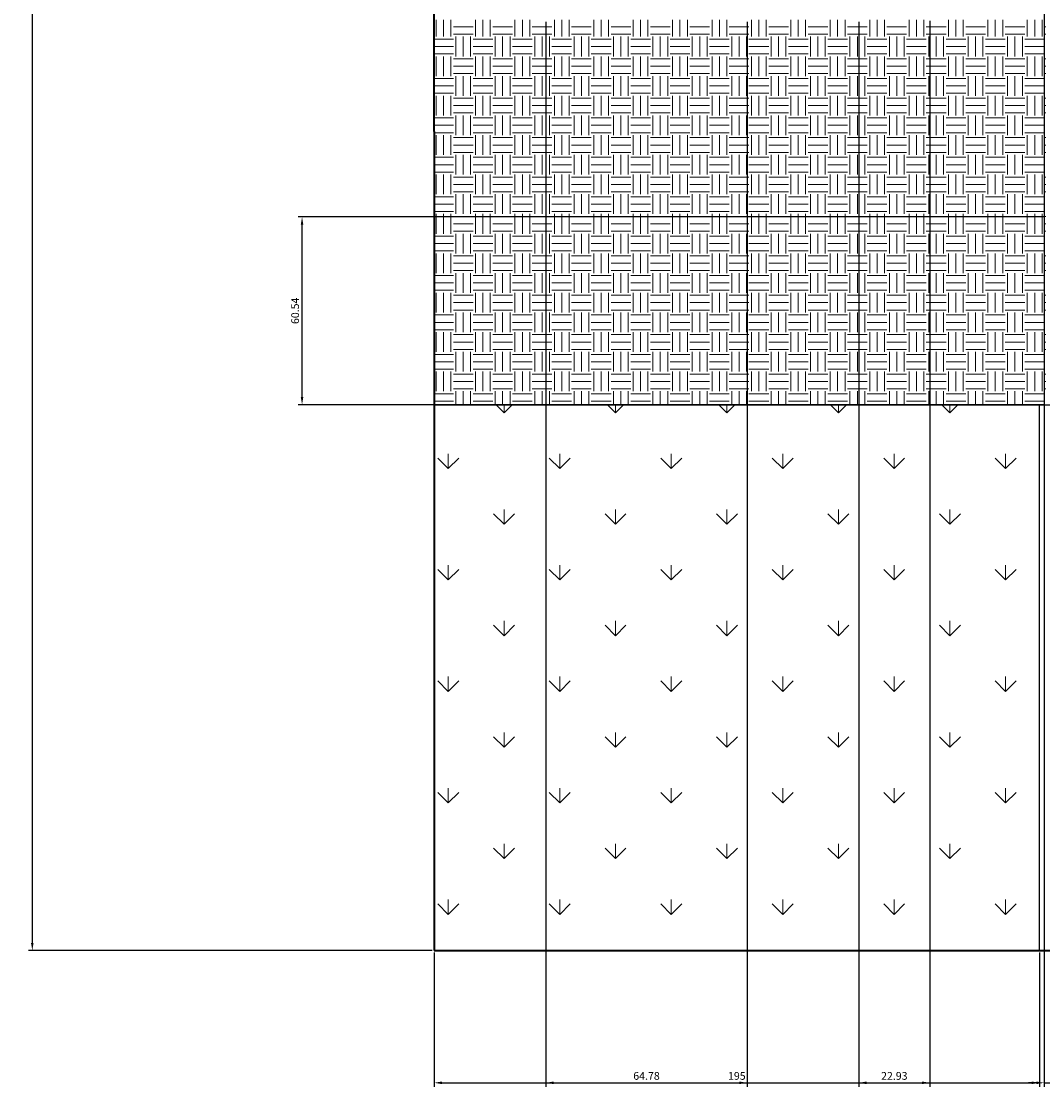
# Model space of a CAD drawing. Units: inches. Extents: x 204 to 942, y 1794 to 2670.
# Tile 1 of 6: x 204 to 533, y 1794 to 2138. Entities that reach past the tile are written whole.
import ezdxf

# ---------------------------------------------------------------- set-up
doc = ezdxf.new("R2010")
doc.units = ezdxf.units.IN
for name, color, linetype, lineweight in [('A-ANNO-DIMS', 2, 'Continuous', 18), ('A-FLOR-OTLN', 7, 'Continuous', 25), ('C-PRKG', 8, 'Continuous', 25), ('C-PROP', 7, 'Continuous', 35)]:
    doc.layers.add(name, color=color, linetype=linetype, lineweight=lineweight)
doc.layers.add('A-FLOR-PATT', color=251, linetype='Continuous', lineweight=13, true_color=0x636466)
doc.layers.add('L-PLNT-PATT', color=85, linetype='Continuous', lineweight=13, true_color=0x58ba48)
doc.styles.get("Standard").update_dxf_attribs({"font": 'arial.ttf'})
doc.dimstyles.new('ISO-25', dxfattribs={"dimtxt": 2.5, "dimasz": 2.5, "dimexe": 1.25, "dimexo": 0.625, "dimtad": 1, "dimtxsty": 'Standard', "dimcen": 2.5, "dimadec": 0, "dimazin": 0, "dimtfac": 1, "dimtmove": 0, "dimatfit": 3, "dimfxl": 1, "dimarcsym": 0})

# ---------------------------------------------------------------- blocks, each defined once
blk = doc.blocks.new('*D11')
at = {"layer": 'A-ANNO-DIMS', "color": 0, "lineweight": -2, "transparency": 16777216}
for p, q in [((336.12, 2624.26), (205.97, 2624.26)), ((207.22, 2621.76), (207.22, 1840.76)), ((336.12, 1838.26), (205.97, 1838.26))]:
    blk.add_line(p, q, dxfattribs=at)
at = {"layer": 'A-ANNO-DIMS', "color": 0, "transparency": 16777216}
for points in [[(206.8, 2621.76), (207.63, 2621.76), (207.22, 2624.26)], [(206.8, 1840.76), (207.63, 1840.76), (207.22, 1838.26)]]:
    blk.add_solid(points, dxfattribs=at)
at = {"layer": 'Defpoints', "color": 0, "transparency": 16777216}
for p in [(336.74, 2624.26), (207.22, 1838.26), (336.74, 1838.26)]:
    blk.add_point(p, dxfattribs=at)
at = {"layer": 'A-ANNO-DIMS', "color": 0, "transparency": 16777216, "insert": (205.32, 2231.26), "char_height": 2.5, "attachment_point": 5, "rotation": 90}
blk.add_mtext('786', dxfattribs=at)
blk = doc.blocks.new('*D44')
at = {"layer": 'A-ANNO-DIMS', "color": 0, "lineweight": -2, "transparency": 16777216}
for p, q in [((336.74, 1837.63), (336.74, 1794.41)), ((531.74, 1837.63), (531.74, 1794.41)), ((339.24, 1795.66), (529.24, 1795.66))]:
    blk.add_line(p, q, dxfattribs=at)
at = {"layer": 'A-ANNO-DIMS', "color": 0, "transparency": 16777216}
for points in [[(339.24, 1796.08), (339.24, 1795.24), (336.74, 1795.66)], [(529.24, 1796.08), (529.24, 1795.24), (531.74, 1795.66)]]:
    blk.add_solid(points, dxfattribs=at)
at = {"layer": 'Defpoints', "color": 0, "transparency": 16777216}
for p in [(336.74, 1838.26), (531.74, 1838.26), (531.74, 1795.66)]:
    blk.add_point(p, dxfattribs=at)
at = {"layer": 'A-ANNO-DIMS', "color": 0, "transparency": 16777216, "insert": (434.24, 1797.56), "char_height": 2.5, "attachment_point": 5}
blk.add_mtext('195', dxfattribs=at)
blk = doc.blocks.new('*D49')
at = {"layer": 'A-ANNO-DIMS', "color": 0, "lineweight": -2, "transparency": 16777216}
for p, q in [((533.24, 2074.72), (292.89, 2074.72)), ((294.14, 2016.68), (294.14, 2072.22)), ((533.24, 2014.18), (292.89, 2014.18))]:
    blk.add_line(p, q, dxfattribs=at)
at = {"layer": 'A-ANNO-DIMS', "color": 0, "transparency": 16777216}
for points in [[(293.73, 2072.22), (294.56, 2072.22), (294.14, 2074.72)], [(293.73, 2016.68), (294.56, 2016.68), (294.14, 2014.18)]]:
    blk.add_solid(points, dxfattribs=at)
at = {"layer": 'Defpoints', "color": 0, "transparency": 16777216}
for p in [(294.14, 2074.72), (533.86, 2074.72), (533.86, 2014.18)]:
    blk.add_point(p, dxfattribs=at)
at = {"layer": 'A-ANNO-DIMS', "color": 0, "transparency": 16777216, "insert": (292.24, 2044.45), "char_height": 2.5, "attachment_point": 5, "rotation": 90}
blk.add_mtext('60.54', dxfattribs=at)
blk = doc.blocks.new('*D50')
at = {"layer": 'A-ANNO-DIMS', "color": 0, "lineweight": -2, "transparency": 16777216}
for p, q in [((533.24, 2587.63), (533.24, 1794.41)), ((537.74, 2578.63), (537.74, 1794.41)), ((530.74, 1795.66), (528.24, 1795.66)), ((533.24, 1795.66), (537.74, 1795.66)), ((540.24, 1795.66), (548.67, 1795.66))]:
    blk.add_line(p, q, dxfattribs=at)
at = {"layer": 'A-ANNO-DIMS', "color": 0, "transparency": 16777216}
for points in [[(530.74, 1796.08), (530.74, 1795.24), (533.24, 1795.66)], [(540.24, 1796.08), (540.24, 1795.24), (537.74, 1795.66)]]:
    blk.add_solid(points, dxfattribs=at)
at = {"layer": 'Defpoints', "color": 0, "transparency": 16777216}
for p in [(533.24, 2588.26), (537.74, 2579.26), (537.74, 1795.66)]:
    blk.add_point(p, dxfattribs=at)
at = {"layer": 'A-ANNO-DIMS', "color": 0, "transparency": 16777216, "insert": (545.7, 1797.56), "char_height": 2.5, "attachment_point": 5}
blk.add_mtext('4.5', dxfattribs=at)
blk = doc.blocks.new('*D54')
at = {"layer": 'A-ANNO-DIMS', "color": 0, "lineweight": -2, "transparency": 16777216}
for p, q in [((372.74, 2137.63), (372.74, 1794.41)), ((437.53, 2137.62), (437.53, 1794.41)), ((375.24, 1795.66), (435.03, 1795.66))]:
    blk.add_line(p, q, dxfattribs=at)
at = {"layer": 'A-ANNO-DIMS', "color": 0, "transparency": 16777216}
for points in [[(375.24, 1796.08), (375.24, 1795.24), (372.74, 1795.66)], [(435.03, 1796.08), (435.03, 1795.24), (437.53, 1795.66)]]:
    blk.add_solid(points, dxfattribs=at)
at = {"layer": 'Defpoints', "color": 0, "transparency": 16777216}
for p in [(372.74, 2138.26), (437.53, 2138.25), (437.53, 1795.66)]:
    blk.add_point(p, dxfattribs=at)
at = {"layer": 'A-ANNO-DIMS', "color": 0, "transparency": 16777216, "insert": (405.14, 1797.56), "char_height": 2.5, "attachment_point": 5}
blk.add_mtext('64.78', dxfattribs=at)
blk = doc.blocks.new('*D55')
at = {"layer": 'A-ANNO-DIMS', "color": 0, "lineweight": -2, "transparency": 16777216}
for p, q in [((473.53, 2137.62), (473.53, 1794.41)), ((496.46, 2137.89), (496.46, 1794.41)), ((476.03, 1795.66), (493.96, 1795.66))]:
    blk.add_line(p, q, dxfattribs=at)
at = {"layer": 'A-ANNO-DIMS', "color": 0, "transparency": 16777216}
for points in [[(476.03, 1796.08), (476.03, 1795.24), (473.53, 1795.66)], [(493.96, 1796.08), (493.96, 1795.24), (496.46, 1795.66)]]:
    blk.add_solid(points, dxfattribs=at)
at = {"layer": 'Defpoints', "color": 0, "transparency": 16777216}
for p in [(473.53, 2138.25), (496.46, 2138.52), (496.46, 1795.66)]:
    blk.add_point(p, dxfattribs=at)
at = {"layer": 'A-ANNO-DIMS', "color": 0, "transparency": 16777216, "insert": (484.99, 1797.56), "char_height": 2.5, "attachment_point": 5}
blk.add_mtext('22.93', dxfattribs=at)

msp = doc.modelspace()

# ---------------------------------------------------------------- hatches: boundary and pattern name
at = {"layer": 'A-FLOR-PATT'}
h = msp.add_hatch(dxfattribs=at)
h.set_pattern_fill('EARTH', color=256)
h.paths.add_polyline_path([(533.8633, 2137.2597), (533.8633, 2138.2597), (473.5284, 2138.2597), (473.5284, 2138.2472), (471.5284, 2138.2472), (437.5284, 2138.2472), (372.7443, 2138.2597), (336.7443, 2138.2597), (336.7443, 2014.1774), (533.8633, 2014.1774)])
at = {"layer": 'L-PLNT-PATT'}
h = msp.add_hatch(dxfattribs=at)
h.set_pattern_fill('GRASS', color=256)
h.paths.add_polyline_path([(531.7443, 2014.1774), (336.7443, 2014.1774), (336.7443, 1838.2597), (531.7443, 1838.2597)])

# ---------------------------------------------------------------- linework, layer by layer
at = {"layer": 'A-FLOR-OTLN'}
for p, q in [((336.7443, 2138.2597), (336.7443, 2014.1774)), ((336.7443, 2014.1774), (545.8757, 2014.1774))]:
    msp.add_line(p, q, dxfattribs=at)
at = {"layer": 'C-PRKG'}
msp.add_line((531.7443, 1838.2597), (531.7443, 2014.1774), dxfattribs=at)
at = {"layer": 'C-PROP'}
for p, q in [((336.7443, 2102.2597), (336.7443, 1838.2597)), ((336.7443, 1838.2597), (726.7443, 1838.2597))]:
    msp.add_line(p, q, dxfattribs=at)
msp.add_lwpolyline([(336.7443, 2102.2597), (336.7443, 2624.2597), (726.7443, 2624.2597), (726.7443, 2102.2597)], dxfattribs=at)

# ---------------------------------------------------------------- dimensions: what is measured, and where the dimension line sits
at = {"layer": 'A-ANNO-DIMS'}
for base, p1, p2, override, picture, middle in [((207.2181, 1838.2597), (336.7443, 2624.2597), (336.7443, 1838.2597), {"dimclrd": 0, "dimclre": 0, "dimclrt": 0}, '*D11', (205.3166, 2231.2597)), ((294.1443, 2074.7185), (533.8633, 2014.1774), (533.8633, 2074.7185), {"dimdec": 2, "dimlfac": 1, "dimrnd": 0, "dimzin": 0, "dimdsep": 46, "dimlunit": 2}, '*D49', (292.2429, 2044.4479))]:
    dim = msp.add_linear_dim(base=base, p1=p1, p2=p2, angle=90, dimstyle='ISO-25', override=override, dxfattribs=at)
    dim.commit()
    dim.dimension.update_dxf_attribs({"geometry": picture, "text_midpoint": middle})
for base, p1, p2, override, picture, middle in [((537.7443, 1795.6597), (533.2443, 2588.2597), (537.7443, 2579.2597), {"dimdec": 1, "dimlfac": 1, "dimrnd": 0, "dimzin": 0, "dimdsep": 46, "dimlunit": 2}, '*D50', (545.7047, 1797.556)), ((437.5284, 1795.6597), (372.7443, 2138.2597), (437.5284, 2138.2472), {"dimdec": 2, "dimlfac": 1, "dimrnd": 0, "dimzin": 0, "dimdsep": 46, "dimlunit": 2}, '*D54', (405.1364, 1797.5611)), ((496.4586, 1795.6597), (473.5284, 2138.2472), (496.4586, 2138.5155), {"dimdec": 2, "dimlfac": 1, "dimrnd": 0, "dimzin": 0, "dimdsep": 46, "dimlunit": 2}, '*D55', (484.9935, 1797.5619)), ((531.7443, 1795.6597), (336.7443, 1838.2597), (531.7443, 1838.2597), {"dimdec": 0, "dimlfac": 1, "dimrnd": 0, "dimzin": 0, "dimdsep": 46, "dimlunit": 2}, '*D44', (434.2443, 1797.5611))]:
    dim = msp.add_linear_dim(base=base, p1=p1, p2=p2, dimstyle='ISO-25', override=override, dxfattribs=at)
    dim.commit()
    dim.dimension.update_dxf_attribs({"geometry": picture, "text_midpoint": middle})

doc.saveas('drawing.dxf')
